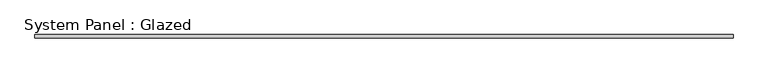
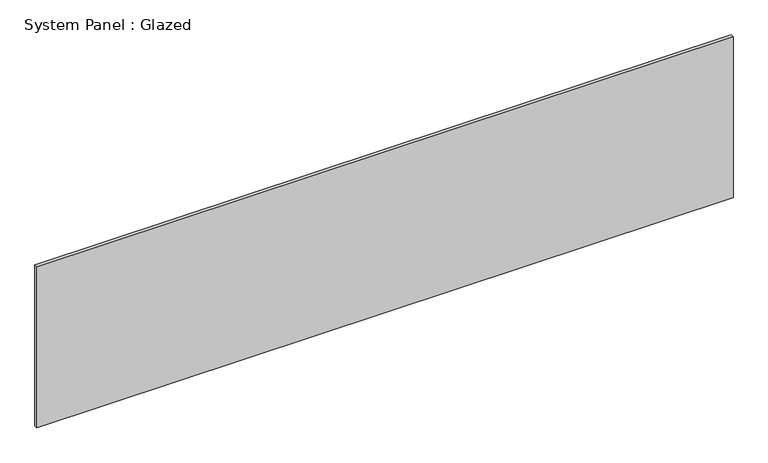
"""IFC4 building model written with IfcOpenShell, lengths in millimetres: plate geometry, System Panel : Glazed."""

from ifc_helpers import new_model, si_unit, origin, origin_with_axes, place, context, project, spatial, polyline, outline, extrude, source, transform, mapped, element, save


def system_panel_glazed_a1141da7(model_context):
    return source(origin(), model_context, "Body", "SweptSolid", [
        extrude(outline(polyline([(2492.8598823, 19.05), (-2492.8598823, 19.05), (-2492.8598823, 44.45), (2492.8598823, 44.45), (2492.8598823, 19.05)])), origin_with_axes(), (0.0, 0.0, 1.0), 1219.2),
    ])


if __name__ == "__main__":
    model = new_model("IFC4")
    model_context = context("Model", 3, world=origin())
    ifc_project = project(units=[si_unit("LENGTHUNIT", "METRE", prefix="MILLI")], contexts=[model_context])
    site = spatial("IfcSite", under=ifc_project)
    building = spatial("IfcBuilding", under=site)
    placement = place(None, origin())
    system_panel_glazed_shape = system_panel_glazed_a1141da7(model_context)
    element("IfcPlate", 1, ObjectType="System Panel : Glazed", at=placement, inside=building, context=model_context, shape_type="MappedRepresentation", body=[
        mapped(system_panel_glazed_shape, transform((0.0, 0.0, 0.0), x_axis=(1.0, 0.0, 0.0), y_axis=(0.0, 1.0, 0.0), z_axis=(0.0, 0.0, 1.0))),
    ])
    save(model, "model.ifc")

# Revit data of these elements
# Type "System Panel : Glazed"
#   Construction Type Id = "GSP4R"
#   Analytic Construction = "1/8 in Pilkington single glazing"
#   Visual Light Transmittance = 0.9
#   Solar Heat Gain Coefficient = 0.86
#   Heat Transfer Coefficient (U) = 1.18115 BTU/(h·ft²·°F)
# Element 1 (IfcPlate, "System Panel : Glazed")
#   Materials on its faces: "Glass"
# Materials
#   "Glass": class "Glass", colour RGB 0 128 192, transparency 0.75, Description = "Soda Lime Glass", Cost = 0
